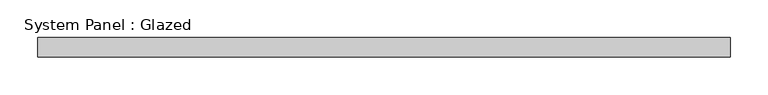
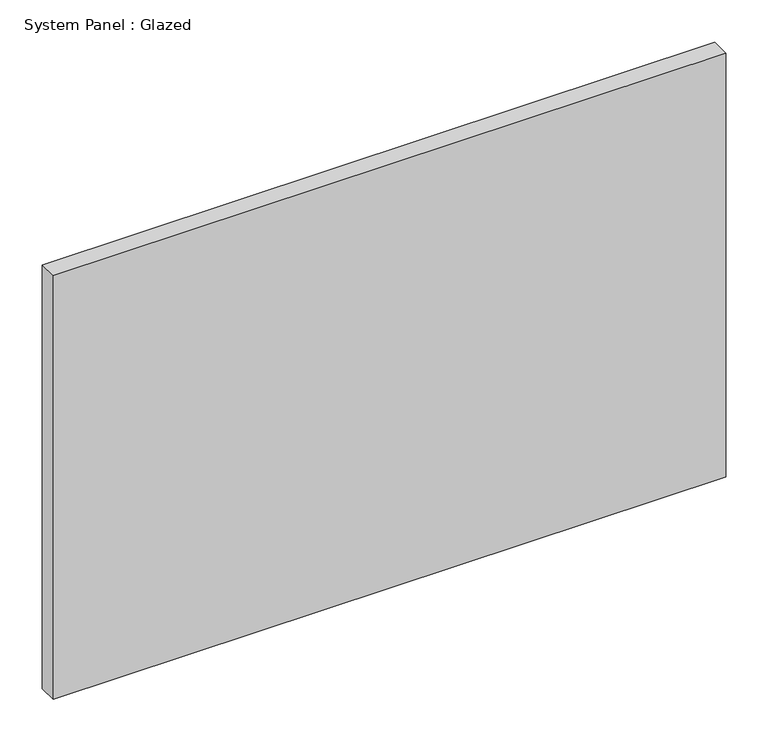
"""IFC4 building model written with IfcOpenShell, lengths in millimetres: plate geometry, System Panel : Glazed."""

from ifc_helpers import new_model, si_unit, origin, origin_with_axes, place, context, project, spatial, polyline, outline, extrude, source, transform, mapped, element, save


def system_panel_glazed_82e05715(model_context):
    return source(origin(), model_context, "Body", "SweptSolid", [
        extrude(outline(polyline([(457.2, 19.05), (-457.2, 19.05), (-457.2, 44.45), (457.2, 44.45), (457.2, 19.05)])), origin_with_axes(), (0.0, 0.0, 1.0), 609.6),
    ])


if __name__ == "__main__":
    model = new_model("IFC4")
    model_context = context("Model", 3, world=origin())
    ifc_project = project(units=[si_unit("LENGTHUNIT", "METRE", prefix="MILLI")], contexts=[model_context])
    site = spatial("IfcSite", under=ifc_project)
    building = spatial("IfcBuilding", under=site)
    placement = place(None, origin())
    system_panel_glazed_shape = system_panel_glazed_82e05715(model_context)
    element("IfcPlate", 1, ObjectType="System Panel : Glazed", at=placement, inside=building, context=model_context, shape_type="MappedRepresentation", body=[
        mapped(system_panel_glazed_shape, transform((0.0, 0.0, 0.0), x_axis=(1.0, 0.0, 0.0), y_axis=(0.0, 1.0, 0.0), z_axis=(0.0, 0.0, 1.0))),
    ])
    save(model, "model.ifc")

# Revit data of these elements
# Type "System Panel : Glazed"
#   Construction Type Id = "GSP4R"
#   Analytic Construction = "1/8 in Pilkington single glazing"
#   Visual Light Transmittance = 0.9
#   Solar Heat Gain Coefficient = 0.86
#   Heat Transfer Coefficient (U) = 1.18115 BTU/(h·ft²·°F)
# Element 1 (IfcPlate, "System Panel : Glazed")
#   Materials on its faces: "Glass"
# Materials
#   "Glass": class "Glass", colour RGB 0 128 192, transparency 0.75, Description = "Soda Lime Glass", Cost = 0
